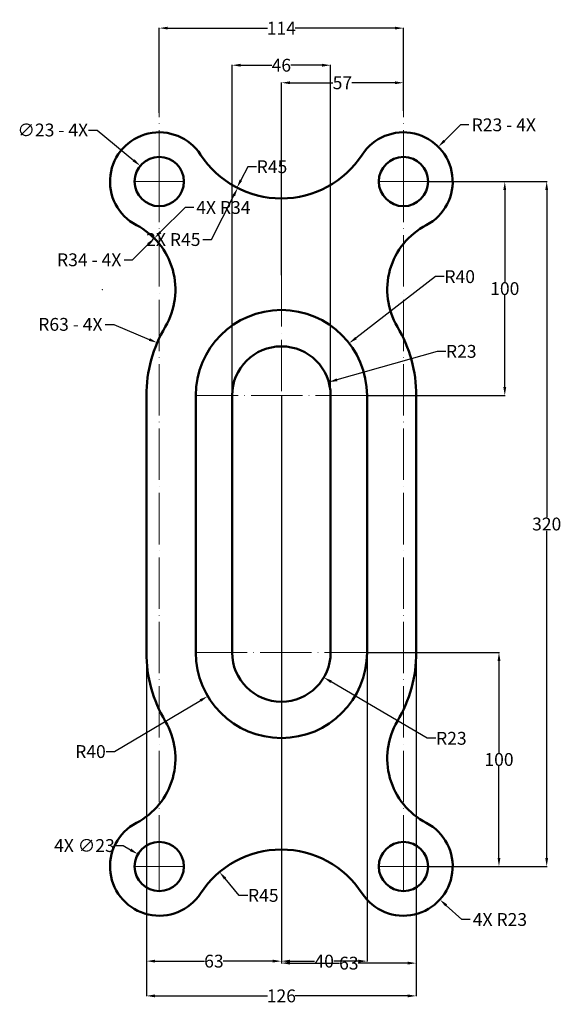
# Model space of a CAD drawing. Units: inches. Extents: x 431 to 684, y 243 to 703.
import ezdxf

# ---------------------------------------------------------------- set-up
doc = ezdxf.new("R2010")
doc.units = ezdxf.units.IN
doc.header["$MEASUREMENT"] = 0
doc.linetypes.add('ACAD_ISO04W100', pattern=[30, 24, -3, 0, -3])
for name, color, linetype, lineweight in [('M-CNTR', 4, 'ACAD_ISO04W100', 18), ('M-DIMS', 2, 'Continuous', 25), ('M-OUTL', 7, 'Continuous', 50)]:
    doc.layers.add(name, color=color, linetype=linetype, lineweight=lineweight)
doc.styles.get("Standard").update_dxf_attribs({"font": 'arial.ttf'})
doc.dimstyles.get("Standard").update_dxf_attribs({"dimtxt": 6, "dimasz": 4, "dimexe": 0.18, "dimexo": 0.0625, "dimgap": 0.09, "dimtad": 0, "dimtih": 1, "dimtoh": 1, "dimdec": 0, "dimzin": 0, "dimdsep": 46, "dimtxsty": 'Standard', "dimcen": 0.09, "dimadec": 0, "dimazin": 0, "dimtfac": 1, "dimtdec": 0, "dimtofl": 0, "dimtmove": 0, "dimatfit": 3, "dimfxl": 1, "dimtolj": 1, "dimtzin": 0, "dimarcsym": 0})

# ---------------------------------------------------------------- blocks, each defined once
blk = doc.blocks.new('*D1')
at = {"layer": 'Defpoints', "color": 0, "transparency": 16777216}
for p in [(622.06, 627.23), (593.56, 527.23), (657.87, 527.23)]:
    blk.add_point(p, dxfattribs=at)
at = {"layer": 'M-DIMS', "color": 0, "lineweight": -2, "transparency": 16777216}
for p, q in [((622.12, 627.23), (658.05, 627.23)), ((657.87, 623.23), (657.87, 580.39)), ((657.87, 531.23), (657.87, 574.08)), ((593.62, 527.23), (658.05, 527.23))]:
    blk.add_line(p, q, dxfattribs=at)
at = {"layer": 'M-DIMS', "color": 0, "transparency": 16777216}
for points in [[(657.2, 623.23), (658.54, 623.23), (657.87, 627.23)], [(657.2, 531.23), (658.54, 531.23), (657.87, 527.23)]]:
    blk.add_solid(points, dxfattribs=at)
at = {"layer": 'M-DIMS', "color": 0, "transparency": 16777216, "insert": (657.87, 577.23), "char_height": 6, "attachment_point": 5}
blk.add_mtext('\\A1;100', dxfattribs=at)
blk = doc.blocks.new('*D2')
at = {"layer": 'Defpoints', "color": 0, "transparency": 16777216}
for p in [(622.06, 627.23), (622.06, 307.23), (677.44, 307.23)]:
    blk.add_point(p, dxfattribs=at)
at = {"layer": 'M-DIMS', "color": 0, "lineweight": -2, "transparency": 16777216}
for p, q in [((622.12, 627.23), (677.62, 627.23)), ((677.44, 623.23), (677.44, 470.39)), ((677.44, 311.23), (677.44, 464.08)), ((622.12, 307.23), (677.62, 307.23))]:
    blk.add_line(p, q, dxfattribs=at)
at = {"layer": 'M-DIMS', "color": 0, "transparency": 16777216}
for points in [[(676.78, 623.23), (678.11, 623.23), (677.44, 627.23)], [(676.78, 311.23), (678.11, 311.23), (677.44, 307.23)]]:
    blk.add_solid(points, dxfattribs=at)
at = {"layer": 'M-DIMS', "color": 0, "transparency": 16777216, "insert": (677.44, 467.23), "char_height": 6, "attachment_point": 5}
blk.add_mtext('\\A1;320', dxfattribs=at)
blk = doc.blocks.new('*D3')
at = {"layer": 'Defpoints', "color": 0, "transparency": 16777216}
for p in [(593.56, 407.23), (655.17, 407.23), (622.06, 307.23)]:
    blk.add_point(p, dxfattribs=at)
at = {"layer": 'M-DIMS', "color": 0, "lineweight": -2, "transparency": 16777216}
for p, q in [((593.62, 407.23), (655.35, 407.23)), ((655.17, 403.23), (655.17, 360.39)), ((655.17, 311.23), (655.17, 354.08)), ((622.12, 307.23), (655.35, 307.23))]:
    blk.add_line(p, q, dxfattribs=at)
at = {"layer": 'M-DIMS', "color": 0, "transparency": 16777216}
for points in [[(654.51, 403.23), (655.84, 403.23), (655.17, 407.23)], [(654.51, 311.23), (655.84, 311.23), (655.17, 307.23)]]:
    blk.add_solid(points, dxfattribs=at)
at = {"layer": 'M-DIMS', "color": 0, "transparency": 16777216, "insert": (655.17, 357.23), "char_height": 6, "attachment_point": 5}
blk.add_mtext('\\A1;100', dxfattribs=at)
blk = doc.blocks.new('*D4')
at = {"layer": 'Defpoints', "color": 0, "transparency": 16777216}
for p in [(553.56, 407.23), (573.38, 395.56)]:
    blk.add_point(p, dxfattribs=at)
at = {"layer": 'M-DIMS', "color": 0, "lineweight": -2, "transparency": 16777216}
for p, q in [((553.47, 407.23), (553.65, 407.23)), ((553.56, 407.14), (553.56, 407.32)), ((621.67, 367.12), (576.82, 393.53)), ((625.67, 367.12), (621.67, 367.12))]:
    blk.add_line(p, q, dxfattribs=at)
at = {"layer": 'M-DIMS', "color": 0, "transparency": 16777216}
blk.add_solid([(577.16, 394.11), (576.48, 392.96), (573.38, 395.56)], dxfattribs=at)
at = {"layer": 'M-DIMS', "color": 0, "transparency": 16777216, "insert": (632.93, 367.12), "char_height": 6, "attachment_point": 5}
blk.add_mtext('\\A1;R23', dxfattribs=at)
blk = doc.blocks.new('*D5')
at = {"layer": 'Defpoints', "color": 0, "transparency": 16777216}
for p in [(553.56, 407.23), (519.18, 386.79)]:
    blk.add_point(p, dxfattribs=at)
at = {"layer": 'M-DIMS', "color": 0, "lineweight": -2, "transparency": 16777216}
for p, q in [((553.47, 407.23), (553.65, 407.23)), ((553.56, 407.14), (553.56, 407.32)), ((475.7, 360.93), (515.74, 384.74)), ((471.7, 360.93), (475.7, 360.93))]:
    blk.add_line(p, q, dxfattribs=at)
at = {"layer": 'M-DIMS', "color": 0, "transparency": 16777216}
blk.add_solid([(515.4, 385.32), (516.08, 384.17), (519.18, 386.79)], dxfattribs=at)
at = {"layer": 'M-DIMS', "color": 0, "transparency": 16777216, "insert": (464.45, 360.93), "char_height": 6, "attachment_point": 5}
blk.add_mtext('\\A1;R40', dxfattribs=at)
blk = doc.blocks.new('*D6')
at = {"layer": 'Defpoints', "color": 0, "transparency": 16777216}
for p in [(524.69, 304.68), (553.56, 270.15)]:
    blk.add_point(p, dxfattribs=at)
at = {"layer": 'M-DIMS', "color": 0, "lineweight": -2, "transparency": 16777216}
for p, q in [((533.85, 293.73), (527.26, 301.61)), ((537.85, 293.73), (533.85, 293.73))]:
    blk.add_line(p, q, dxfattribs=at)
at = {"layer": 'M-DIMS', "color": 0, "transparency": 16777216}
blk.add_solid([(527.77, 302.04), (526.75, 301.18), (524.69, 304.68)], dxfattribs=at)
at = {"layer": 'M-DIMS', "color": 0, "transparency": 16777216, "insert": (545.13, 293.73), "char_height": 6, "attachment_point": 5}
blk.add_mtext('\\A1;R45', dxfattribs=at)
blk = doc.blocks.new('*D7')
at = {"layer": 'Defpoints', "color": 0, "transparency": 16777216}
for p in [(616.56, 407.23), (553.56, 354.41), (616.56, 262.08)]:
    blk.add_point(p, dxfattribs=at)
at = {"layer": 'M-DIMS', "color": 0, "lineweight": -2, "transparency": 16777216}
for p, q in [((616.56, 407.17), (616.56, 261.9)), ((553.56, 354.35), (553.56, 261.9)), ((557.56, 262.08), (580.65, 262.08)), ((612.56, 262.08), (589.46, 262.08))]:
    blk.add_line(p, q, dxfattribs=at)
at = {"layer": 'M-DIMS', "color": 0, "transparency": 16777216}
for points in [[(557.56, 262.75), (557.56, 261.42), (553.56, 262.08)], [(612.56, 262.75), (612.56, 261.42), (616.56, 262.08)]]:
    blk.add_solid(points, dxfattribs=at)
at = {"layer": 'M-DIMS', "color": 0, "transparency": 16777216, "insert": (585.06, 262.08), "char_height": 6, "attachment_point": 5}
blk.add_mtext('\\A1;63', dxfattribs=at)
blk = doc.blocks.new('*D8')
at = {"layer": 'Defpoints', "color": 0, "transparency": 16777216}
for p in [(490.56, 407.23), (616.56, 407.23), (616.56, 246.78)]:
    blk.add_point(p, dxfattribs=at)
at = {"layer": 'M-DIMS', "color": 0, "lineweight": -2, "transparency": 16777216}
for p, q in [((490.56, 407.17), (490.56, 246.6)), ((616.56, 407.17), (616.56, 246.6)), ((494.56, 246.78), (547.12, 246.78)), ((612.56, 246.78), (559.99, 246.78))]:
    blk.add_line(p, q, dxfattribs=at)
at = {"layer": 'M-DIMS', "color": 0, "transparency": 16777216}
for points in [[(494.56, 247.45), (494.56, 246.11), (490.56, 246.78)], [(612.56, 247.45), (612.56, 246.11), (616.56, 246.78)]]:
    blk.add_solid(points, dxfattribs=at)
at = {"layer": 'M-DIMS', "color": 0, "transparency": 16777216, "insert": (553.56, 246.78), "char_height": 6, "attachment_point": 5}
blk.add_mtext('\\A1;126', dxfattribs=at)
blk = doc.blocks.new('*D9')
at = {"layer": 'Defpoints', "color": 0, "transparency": 16777216}
for p in [(495.59, 551.9), (553.56, 527.23)]:
    blk.add_point(p, dxfattribs=at)
at = {"layer": 'M-DIMS', "color": 0, "lineweight": -2, "transparency": 16777216}
for p, q in [((471.34, 560.51), (475.34, 560.51)), ((475.34, 560.51), (491.91, 553.47)), ((553.47, 527.23), (553.65, 527.23)), ((553.56, 527.14), (553.56, 527.32))]:
    blk.add_line(p, q, dxfattribs=at)
at = {"layer": 'M-DIMS', "color": 0, "transparency": 16777216}
blk.add_solid([(492.17, 554.08), (491.64, 552.85), (495.59, 551.9)], dxfattribs=at)
at = {"layer": 'M-DIMS', "color": 0, "transparency": 16777216, "insert": (455.07, 560.51), "char_height": 6, "attachment_point": 5}
blk.add_mtext('\\A1;R63 - 4X', dxfattribs=at)
blk = doc.blocks.new('*D10')
at = {"layer": 'Defpoints', "color": 0, "transparency": 16777216}
for p in [(494.2, 600.74), (470.13, 576.73)]:
    blk.add_point(p, dxfattribs=at)
at = {"layer": 'M-DIMS', "color": 0, "lineweight": -2, "transparency": 16777216}
for p, q in [((484.12, 590.68), (491.37, 597.92)), ((480.12, 590.68), (484.12, 590.68))]:
    blk.add_line(p, q, dxfattribs=at)
at = {"layer": 'M-DIMS', "color": 0, "transparency": 16777216}
blk.add_solid([(490.9, 598.39), (491.84, 597.45), (494.2, 600.74)], dxfattribs=at)
at = {"layer": 'M-DIMS', "color": 0, "transparency": 16777216, "insert": (463.84, 590.68), "char_height": 6, "attachment_point": 5}
blk.add_mtext('\\A1;R34 - 4X', dxfattribs=at)
blk = doc.blocks.new('*D11')
at = {"layer": 'Defpoints', "color": 0, "transparency": 16777216}
for p in [(626.85, 643.46), (610.56, 627.23)]:
    blk.add_point(p, dxfattribs=at)
at = {"layer": 'M-DIMS', "color": 0, "lineweight": -2, "transparency": 16777216}
for p, q in [((637.15, 653.72), (629.69, 646.29)), ((641.15, 653.72), (637.15, 653.72)), ((610.47, 627.23), (610.65, 627.23)), ((610.56, 627.14), (610.56, 627.32))]:
    blk.add_line(p, q, dxfattribs=at)
at = {"layer": 'M-DIMS', "color": 0, "transparency": 16777216}
blk.add_solid([(629.22, 646.76), (630.16, 645.81), (626.85, 643.46)], dxfattribs=at)
at = {"layer": 'M-DIMS', "color": 0, "transparency": 16777216, "insert": (657.42, 653.72), "char_height": 6, "attachment_point": 5}
blk.add_mtext('\\A1;R23 - 4X', dxfattribs=at)
blk = doc.blocks.new('*D12')
at = {"layer": 'Defpoints', "color": 0, "transparency": 16777216}
for p in [(553.56, 664.31), (532.84, 624.37)]:
    blk.add_point(p, dxfattribs=at)
at = {"layer": 'M-DIMS', "color": 0, "lineweight": -2, "transparency": 16777216}
for p, q in [((537.91, 634.15), (534.68, 627.92)), ((541.91, 634.15), (537.91, 634.15))]:
    blk.add_line(p, q, dxfattribs=at)
at = {"layer": 'M-DIMS', "color": 0, "transparency": 16777216}
blk.add_solid([(534.09, 628.22), (535.27, 627.61), (532.84, 624.37)], dxfattribs=at)
at = {"layer": 'M-DIMS', "color": 0, "transparency": 16777216, "insert": (549.19, 634.15), "char_height": 6, "attachment_point": 5}
blk.add_mtext('\\A1;R45', dxfattribs=at)
blk = doc.blocks.new('*D13')
at = {"layer": 'Defpoints', "color": 0, "transparency": 16777216}
for p in [(487.7, 634.57), (505.41, 619.89)]:
    blk.add_point(p, dxfattribs=at)
at = {"layer": 'M-DIMS', "color": 0, "lineweight": -2, "transparency": 16777216}
for p, q in [((463.51, 651.31), (467.51, 651.31)), ((467.51, 651.31), (484.62, 637.13)), ((496.47, 627.23), (496.65, 627.23)), ((496.56, 627.14), (496.56, 627.32))]:
    blk.add_line(p, q, dxfattribs=at)
at = {"layer": 'M-DIMS', "color": 0, "transparency": 16777216}
blk.add_solid([(485.05, 637.64), (484.2, 636.61), (487.7, 634.57)], dxfattribs=at)
at = {"layer": 'M-DIMS', "color": 0, "transparency": 16777216, "insert": (446.85, 651.31), "char_height": 6, "attachment_point": 5}
blk.add_mtext('\\A1;∅23 - 4X', dxfattribs=at)
blk = doc.blocks.new('*D14')
at = {"layer": 'Defpoints', "color": 0, "transparency": 16777216}
for p in [(610.56, 698.91), (496.56, 659.31), (610.56, 660.28)]:
    blk.add_point(p, dxfattribs=at)
at = {"layer": 'M-DIMS', "color": 0, "lineweight": -2, "transparency": 16777216}
for p, q in [((496.56, 659.38), (496.56, 699.09)), ((500.56, 698.91), (547.13, 698.91)), ((606.56, 698.91), (559.98, 698.91)), ((610.56, 660.34), (610.56, 699.09))]:
    blk.add_line(p, q, dxfattribs=at)
at = {"layer": 'M-DIMS', "color": 0, "transparency": 16777216}
for points in [[(500.56, 699.58), (500.56, 698.25), (496.56, 698.91)], [(606.56, 699.58), (606.56, 698.25), (610.56, 698.91)]]:
    blk.add_solid(points, dxfattribs=at)
at = {"layer": 'M-DIMS', "color": 0, "transparency": 16777216, "insert": (553.56, 698.91), "char_height": 6, "attachment_point": 5}
blk.add_mtext('\\A1;114', dxfattribs=at)
blk = doc.blocks.new('*D15')
at = {"layer": 'Defpoints', "color": 0, "transparency": 16777216}
for p in [(610.56, 673.39), (610.56, 660.28), (553.56, 583.44)]:
    blk.add_point(p, dxfattribs=at)
at = {"layer": 'M-DIMS', "color": 0, "lineweight": -2, "transparency": 16777216}
for p, q in [((553.56, 583.5), (553.56, 673.57)), ((557.56, 673.39), (577.67, 673.39)), ((606.56, 673.39), (586.44, 673.39)), ((610.56, 660.34), (610.56, 673.57))]:
    blk.add_line(p, q, dxfattribs=at)
at = {"layer": 'M-DIMS', "color": 0, "transparency": 16777216}
for points in [[(557.56, 674.06), (557.56, 672.73), (553.56, 673.39)], [(606.56, 674.06), (606.56, 672.73), (610.56, 673.39)]]:
    blk.add_solid(points, dxfattribs=at)
at = {"layer": 'M-DIMS', "color": 0, "transparency": 16777216, "insert": (582.06, 673.39), "char_height": 6, "attachment_point": 5}
blk.add_mtext('\\A1;57', dxfattribs=at)
blk = doc.blocks.new('*D16')
at = {"layer": 'Defpoints', "color": 0, "transparency": 16777216}
for p in [(585.22, 551.68), (553.56, 527.23)]:
    blk.add_point(p, dxfattribs=at)
at = {"layer": 'M-DIMS', "color": 0, "lineweight": -2, "transparency": 16777216}
for p, q in [((625.57, 582.82), (588.39, 554.12)), ((629.57, 582.82), (625.57, 582.82)), ((553.47, 527.23), (553.65, 527.23)), ((553.56, 527.14), (553.56, 527.32))]:
    blk.add_line(p, q, dxfattribs=at)
at = {"layer": 'M-DIMS', "color": 0, "transparency": 16777216}
blk.add_solid([(587.98, 554.65), (588.79, 553.59), (585.22, 551.68)], dxfattribs=at)
at = {"layer": 'M-DIMS', "color": 0, "transparency": 16777216, "insert": (636.82, 582.82), "char_height": 6, "attachment_point": 5}
blk.add_mtext('\\A1;R40', dxfattribs=at)
blk = doc.blocks.new('*D17')
at = {"layer": 'Defpoints', "color": 0, "transparency": 16777216}
for p in [(575.68, 533.52), (553.56, 527.23)]:
    blk.add_point(p, dxfattribs=at)
at = {"layer": 'M-DIMS', "color": 0, "lineweight": -2, "transparency": 16777216}
for p, q in [((626.29, 547.89), (579.53, 534.61)), ((630.29, 547.89), (626.29, 547.89)), ((553.47, 527.23), (553.65, 527.23)), ((553.56, 527.14), (553.56, 527.32))]:
    blk.add_line(p, q, dxfattribs=at)
at = {"layer": 'M-DIMS', "color": 0, "transparency": 16777216}
blk.add_solid([(579.35, 535.25), (579.71, 533.97), (575.68, 533.52)], dxfattribs=at)
at = {"layer": 'M-DIMS', "color": 0, "transparency": 16777216, "insert": (637.55, 547.89), "char_height": 6, "attachment_point": 5}
blk.add_mtext('\\A1;R23', dxfattribs=at)
blk = doc.blocks.new('ANCHOR-HOLE-D23')
blk.add_circle((0, 0), 11.5)
blk = doc.blocks.new('*D19')
at = {"layer": 'Defpoints', "color": 0, "transparency": 16777216}
for p in [(553.56, 527.23), (593.56, 527.23), (593.56, 263.01)]:
    blk.add_point(p, dxfattribs=at)
at = {"layer": 'M-DIMS', "color": 0, "lineweight": -2, "transparency": 16777216}
for p, q in [((553.56, 527.17), (553.56, 262.83)), ((593.56, 527.17), (593.56, 262.83)), ((557.56, 263.01), (569.06, 263.01)), ((589.56, 263.01), (578.05, 263.01))]:
    blk.add_line(p, q, dxfattribs=at)
at = {"layer": 'M-DIMS', "color": 0, "transparency": 16777216}
for points in [[(557.56, 263.68), (557.56, 262.35), (553.56, 263.01)], [(589.56, 263.68), (589.56, 262.35), (593.56, 263.01)]]:
    blk.add_solid(points, dxfattribs=at)
at = {"layer": 'M-DIMS', "color": 0, "transparency": 16777216, "insert": (573.56, 263.01), "char_height": 6, "attachment_point": 5}
blk.add_mtext('\\A1;40', dxfattribs=at)
blk = doc.blocks.new('*D20')
at = {"layer": 'Defpoints', "color": 0, "transparency": 16777216}
for p in [(576.56, 681.58), (530.56, 407.23), (576.56, 407.23)]:
    blk.add_point(p, dxfattribs=at)
at = {"layer": 'M-DIMS', "color": 0, "lineweight": -2, "transparency": 16777216}
for p, q in [((530.56, 407.3), (530.56, 681.76)), ((534.56, 681.58), (549.05, 681.58)), ((572.56, 681.58), (558.06, 681.58)), ((576.56, 407.3), (576.56, 681.76))]:
    blk.add_line(p, q, dxfattribs=at)
at = {"layer": 'M-DIMS', "color": 0, "transparency": 16777216}
for points in [[(534.56, 682.25), (534.56, 680.92), (530.56, 681.58)], [(572.56, 682.25), (572.56, 680.92), (576.56, 681.58)]]:
    blk.add_solid(points, dxfattribs=at)
at = {"layer": 'M-DIMS', "color": 0, "transparency": 16777216, "insert": (553.56, 681.58), "char_height": 6, "attachment_point": 5}
blk.add_mtext('\\A1;46', dxfattribs=at)
blk = doc.blocks.new('*D21')
at = {"layer": 'Defpoints', "color": 0, "transparency": 16777216}
for p in [(490.56, 527.23), (553.56, 527.23), (553.56, 263.01)]:
    blk.add_point(p, dxfattribs=at)
at = {"layer": 'M-DIMS', "color": 0, "lineweight": -2, "transparency": 16777216}
for p, q in [((490.56, 527.17), (490.56, 262.83)), ((553.56, 527.17), (553.56, 262.83)), ((494.56, 263.01), (517.65, 263.01)), ((549.56, 263.01), (526.46, 263.01))]:
    blk.add_line(p, q, dxfattribs=at)
at = {"layer": 'M-DIMS', "color": 0, "transparency": 16777216}
for points in [[(494.56, 263.68), (494.56, 262.35), (490.56, 263.01)], [(549.56, 263.68), (549.56, 262.35), (553.56, 263.01)]]:
    blk.add_solid(points, dxfattribs=at)
at = {"layer": 'M-DIMS', "color": 0, "transparency": 16777216, "insert": (522.06, 263.01), "char_height": 6, "attachment_point": 5}
blk.add_mtext('\\A1;63', dxfattribs=at)
blk = doc.blocks.new('*D22')
at = {"layer": 'Defpoints', "color": 0, "transparency": 16777216}
for p in [(486.61, 313), (506.51, 301.47)]:
    blk.add_point(p, dxfattribs=at)
at = {"layer": 'M-DIMS', "color": 0, "lineweight": -2, "transparency": 16777216}
for p, q in [((475.68, 317.01), (479.68, 317.01)), ((479.68, 317.01), (483.14, 315)), ((496.47, 307.23), (496.65, 307.23)), ((496.56, 307.14), (496.56, 307.32))]:
    blk.add_line(p, q, dxfattribs=at)
at = {"layer": 'M-DIMS', "color": 0, "transparency": 16777216}
blk.add_solid([(483.48, 315.58), (482.81, 314.42), (486.61, 313)], dxfattribs=at)
at = {"layer": 'M-DIMS', "color": 0, "transparency": 16777216, "insert": (461.62, 317.01), "char_height": 6, "attachment_point": 5}
blk.add_mtext('\\A1;4X ∅23', dxfattribs=at)
blk = doc.blocks.new('*D23')
at = {"layer": 'Defpoints', "color": 0, "transparency": 16777216}
for p in [(610.56, 307.23), (627.57, 291.76)]:
    blk.add_point(p, dxfattribs=at)
at = {"layer": 'M-DIMS', "color": 0, "lineweight": -2, "transparency": 16777216}
for p, q in [((610.47, 307.23), (610.65, 307.23)), ((610.56, 307.14), (610.56, 307.32)), ((637.78, 282.47), (630.53, 289.07)), ((641.78, 282.47), (637.78, 282.47))]:
    blk.add_line(p, q, dxfattribs=at)
at = {"layer": 'M-DIMS', "color": 0, "transparency": 16777216}
blk.add_solid([(630.98, 289.56), (630.08, 288.57), (627.57, 291.76)], dxfattribs=at)
at = {"layer": 'M-DIMS', "color": 0, "transparency": 16777216, "insert": (655.61, 282.47), "char_height": 6, "attachment_point": 5}
blk.add_mtext('\\A1;4X R23', dxfattribs=at)
blk = doc.blocks.new('*D24')
at = {"layer": 'Defpoints', "color": 0, "transparency": 16777216}
for p in [(553.56, 664.31), (533.15, 624.21)]:
    blk.add_point(p, dxfattribs=at)
at = {"layer": 'M-DIMS', "color": 0, "lineweight": -2, "transparency": 16777216}
for p, q in [((553.47, 664.31), (553.65, 664.31)), ((553.56, 664.22), (553.56, 664.4)), ((520.91, 600.14), (531.34, 620.64)), ((516.91, 600.14), (520.91, 600.14))]:
    blk.add_line(p, q, dxfattribs=at)
at = {"layer": 'M-DIMS', "color": 0, "transparency": 16777216}
blk.add_solid([(530.75, 620.94), (531.93, 620.34), (533.15, 624.21)], dxfattribs=at)
at = {"layer": 'M-DIMS', "color": 0, "transparency": 16777216, "insert": (503.13, 600.14), "char_height": 6, "attachment_point": 5}
blk.add_mtext('\\A1;2X R45', dxfattribs=at)
blk = doc.blocks.new('*D25')
at = {"layer": 'Defpoints', "color": 0, "transparency": 16777216}
for p in [(494.22, 600.72), (470.13, 576.73)]:
    blk.add_point(p, dxfattribs=at)
at = {"layer": 'M-DIMS', "color": 0, "lineweight": -2, "transparency": 16777216}
for p, q in [((508.68, 615.12), (497.06, 603.54)), ((512.68, 615.12), (508.68, 615.12)), ((470.04, 576.73), (470.22, 576.73)), ((470.13, 576.64), (470.13, 576.82))]:
    blk.add_line(p, q, dxfattribs=at)
at = {"layer": 'M-DIMS', "color": 0, "transparency": 16777216}
blk.add_solid([(496.59, 604.02), (497.53, 603.07), (494.22, 600.72)], dxfattribs=at)
at = {"layer": 'M-DIMS', "color": 0, "transparency": 16777216, "insert": (526.49, 615.12), "char_height": 6, "attachment_point": 5}
blk.add_mtext('\\A1;4X R34', dxfattribs=at)

msp = doc.modelspace()

# ---------------------------------------------------------------- linework, layer by layer
at = {"layer": 'M-CNTR'}
for p, q in [((485.06, 627.23), (508.06, 627.23)), ((599.06, 627.23), (622.06, 627.23)), ((553.56, 583.44), (553.56, 354.41)), ((593.56, 527.23), (513.56, 527.23)), ((513.56, 407.23), (593.56, 407.23)), ((485.06, 307.23), (508.06, 307.23)), ((599.06, 307.23), (622.06, 307.23))]:
    msp.add_line(p, q, dxfattribs=at)
for points in [[(496.56, 295.73), (496.56, 307.23), (496.56, 627.23), (496.56, 659.31)], [(610.56, 295.73), (610.56, 307.23), (610.56, 627.23), (610.56, 660.28)]]:
    msp.add_lwpolyline(points, dxfattribs=at)
at = {"layer": 'M-OUTL'}
for p, q in [((490.56, 407.23), (490.56, 527.23)), ((513.56, 407.23), (513.56, 527.23)), ((530.56, 407.23), (530.56, 527.23)), ((576.56, 407.23), (576.56, 527.23)), ((593.56, 407.23), (593.56, 527.23)), ((616.56, 407.23), (616.56, 527.23))]:
    msp.add_line(p, q, dxfattribs=at)
for centre, radius, start, end in [((496.56, 627.23), 23, 33.0458, 242.3833), ((610.56, 627.23), 23, 297.6167, 146.9542), ((553.56, 664.31), 45, 213.0458, 326.9542), ((470.13, 576.73), 34, 329.3196, 62.3833), ((636.98, 576.73), 34, 117.6167, 210.6804), ((553.56, 527.23), 40, 0, 180), ((553.56, 527.23), 63, 149.3196, 180), ((553.56, 527.23), 63, 0, 30.6804), ((553.56, 527.23), 23, 0, 180), ((553.56, 407.23), 63, 180, 210.6804), ((553.56, 407.23), 40, 180, 0), ((553.56, 407.23), 23, 180, 0), ((553.56, 407.23), 63, 329.3196, 0), ((470.13, 357.74), 34, 297.6167, 30.6804), ((636.98, 357.74), 34, 149.3196, 242.3833), ((496.56, 307.23), 23, 117.6167, 326.9542), ((610.56, 307.23), 23, 213.0458, 62.3833), ((553.56, 270.15), 45, 33.0458, 146.9542)]:
    msp.add_arc(centre, radius, start, end, dxfattribs=at)

# ---------------------------------------------------------------- block references
for p in [(496.56, 627.23), (610.56, 627.23), (496.56, 307.23), (610.56, 307.23)]:
    msp.add_blockref('ANCHOR-HOLE-D23', p, dxfattribs=at)

# ---------------------------------------------------------------- dimensions: what is measured, and where the dimension line sits
at = {"layer": 'M-DIMS'}
for base, p1, p2, override, picture, middle in [((610.56, 698.91), (496.56, 659.31), (610.56, 660.28), {"dimclrd": 0, "dimclre": 0, "dimclrt": 0}, '*D14', (553.56, 698.91)), ((576.56, 681.58), (530.56, 407.23), (576.56, 407.23), {"dimdec": 0, "dimlfac": 1, "dimrnd": 0, "dimzin": 0, "dimdsep": 46, "dimlunit": 2}, '*D20', (553.56, 681.58)), ((610.56, 673.39), (553.56, 583.44), (610.56, 660.28), {"dimclrd": 0, "dimclre": 0, "dimclrt": 0}, '*D15', (582.06, 673.39)), ((553.56, 263.01), (490.56, 527.23), (553.56, 527.23), {"dimdec": 0, "dimlfac": 1, "dimrnd": 0, "dimzin": 0, "dimdsep": 46, "dimlunit": 2}, '*D21', (522.06, 263.01)), ((593.56, 263.01), (553.56, 527.23), (593.56, 527.23), {"dimdec": 0, "dimlfac": 1, "dimrnd": 0, "dimzin": 0, "dimdsep": 46, "dimlunit": 2}, '*D19', (573.56, 263.01)), ((616.56, 246.78), (490.56, 407.23), (616.56, 407.23), {"dimclrd": 0, "dimclre": 0, "dimclrt": 0}, '*D8', (553.56, 246.78)), ((616.56, 262.08), (553.56, 354.41), (616.56, 407.23), {"dimclrd": 0, "dimclre": 0, "dimclrt": 0}, '*D7', (585.06, 262.08))]:
    dim = msp.add_linear_dim(base=base, p1=p1, p2=p2, dimstyle='Standard', override=override, dxfattribs=at)
    dim.commit()
    dim.dimension.update_dxf_attribs({"geometry": picture, "text_midpoint": middle})
for center, mpoint, text, override, picture, middle in [((610.56, 627.23), (626.85, 643.46), '<> - 4X', {"dimclrd": 0, "dimclre": 0, "dimclrt": 0}, '*D11', (657.42, 653.72)), ((553.56, 664.31), (533.15, 624.21), '2X <>', {"dimdec": 0, "dimlfac": 1, "dimrnd": 0, "dimzin": 0, "dimdsep": 46, "dimlunit": 2}, '*D24', (503.13, 600.14)), ((470.13, 576.73), (494.22, 600.72), '4X <>', {"dimdec": 0, "dimlfac": 1, "dimrnd": 0, "dimzin": 0, "dimdsep": 46, "dimlunit": 2}, '*D25', (526.49, 615.12)), ((470.13, 576.73), (494.2, 600.74), '<> - 4X', {"dimclrd": 0, "dimclre": 0, "dimclrt": 0}, '*D10', (463.84, 590.68)), ((553.56, 527.23), (495.59, 551.9), '<> - 4X', {"dimclrd": 0, "dimclre": 0, "dimclrt": 0}, '*D9', (455.07, 560.51)), ((610.56, 307.23), (627.57, 291.76), '4X <>', {"dimdec": 0, "dimlfac": 1, "dimrnd": 0, "dimzin": 0, "dimdsep": 46, "dimlunit": 2}, '*D23', (655.61, 282.47))]:
    dim = msp.add_radius_dim(center=center, mpoint=mpoint, text=text, dimstyle='Standard', override=override, dxfattribs=at)
    dim.commit()
    dim.dimension.update_dxf_attribs({"geometry": picture, "text_midpoint": middle, "dimtype": 164})
for p1, p2, text, override, picture, middle in [((505.41, 619.89), (487.7, 634.57), '<> - 4X', {"dimclrd": 0, "dimclre": 0, "dimclrt": 0}, '*D13', (446.85, 651.31)), ((506.51, 301.47), (486.61, 313), '4X <>', {"dimdec": 0, "dimlfac": 1, "dimrnd": 0, "dimzin": 0, "dimdsep": 46, "dimlunit": 2}, '*D22', (461.62, 317.01))]:
    dim = msp.add_diameter_dim_2p(p1=p1, p2=p2, text=text, dimstyle='Standard', override=override, dxfattribs=at)
    dim.commit()
    dim.dimension.update_dxf_attribs({"geometry": picture, "text_midpoint": middle, "dimtype": 163})
for center, mpoint, picture, middle in [((553.56, 664.31), (532.84, 624.37), '*D12', (549.19, 634.15)), ((553.56, 527.23), (585.22, 551.68), '*D16', (636.82, 582.82)), ((553.56, 527.23), (575.68, 533.52), '*D17', (637.55, 547.89)), ((553.56, 407.23), (519.18, 386.79), '*D5', (464.45, 360.93)), ((553.56, 407.23), (573.38, 395.56), '*D4', (632.93, 367.12)), ((553.56, 270.15), (524.69, 304.68), '*D6', (545.13, 293.73))]:
    dim = msp.add_radius_dim(center=center, mpoint=mpoint, dimstyle='Standard', override={"dimclrd": 0, "dimclre": 0, "dimclrt": 0}, dxfattribs=at)
    dim.commit()
    dim.dimension.update_dxf_attribs({"geometry": picture, "text_midpoint": middle, "dimtype": 164})
for base, p1, p2, picture, middle in [((657.87, 527.23), (622.06, 627.23), (593.56, 527.23), '*D1', (657.87, 577.23)), ((677.44, 307.23), (622.06, 627.23), (622.06, 307.23), '*D2', (677.44, 467.23)), ((655.17, 407.23), (622.06, 307.23), (593.56, 407.23), '*D3', (655.17, 357.23))]:
    dim = msp.add_linear_dim(base=base, p1=p1, p2=p2, angle=90, dimstyle='Standard', override={"dimclrd": 0, "dimclre": 0, "dimclrt": 0}, dxfattribs=at)
    dim.commit()
    dim.dimension.update_dxf_attribs({"geometry": picture, "text_midpoint": middle})

doc.saveas('drawing.dxf')
